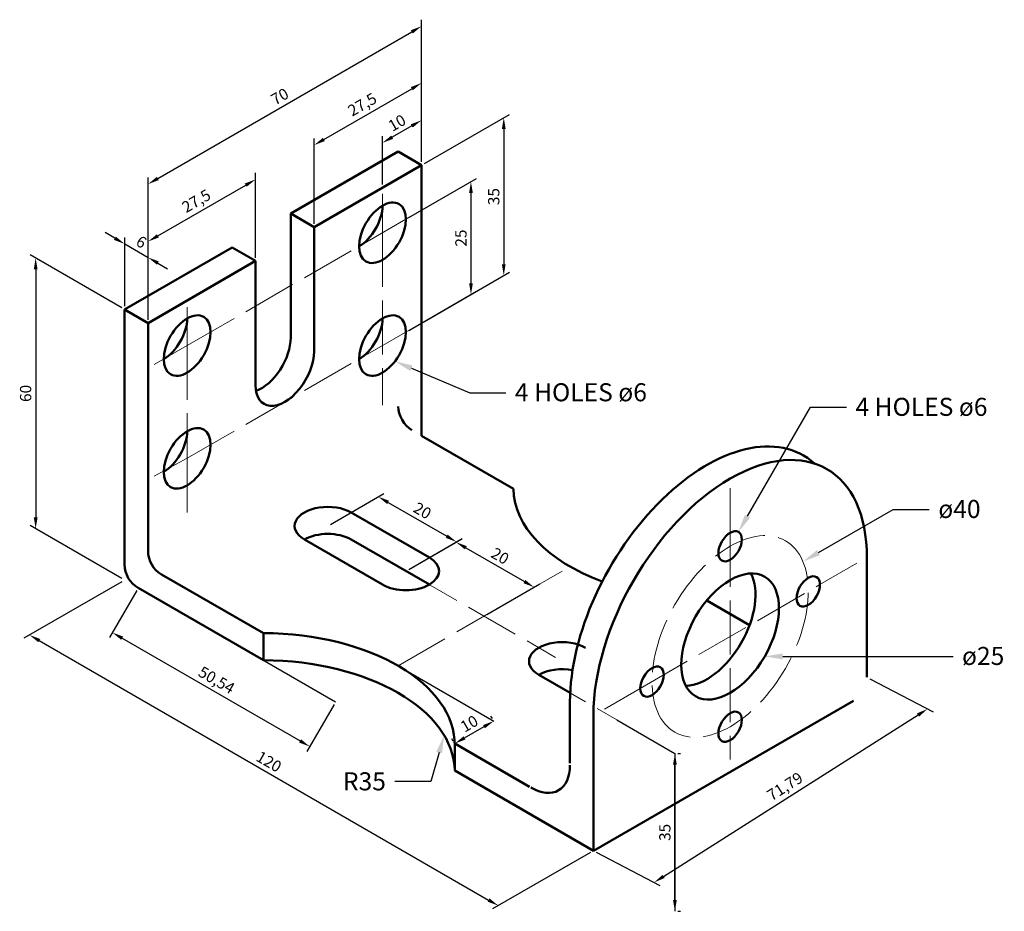
# Model space of a CAD drawing. Units: millimetres. Extents: x 1305 to 1523, y 1896 to 2094.
import ezdxf
from ezdxf import colors
from ezdxf.entities.mleader import LeaderData, LeaderLine
from ezdxf.math import Vec2, Vec3

# ---------------------------------------------------------------- set-up
doc = ezdxf.new("R2010")
doc.units = ezdxf.units.MM
doc.linetypes.add('ACAD_ISO02W100', pattern=[15, 12, -3])
for name, color, linetype, lineweight in [('M-CNTR', 1, 'ACAD_ISO02W100', 18), ('M-DIMS', 2, 'Continuous', 25), ('M-OUTL', 7, 'Continuous', 50), ('M-TEXT', 3, 'Continuous', 25)]:
    doc.layers.add(name, color=color, linetype=linetype, lineweight=lineweight)
doc.styles.get("Standard").update_dxf_attribs({"font": 'arial.ttf'})
doc.dimstyles.new('ISO-25', dxfattribs={"dimtxt": 2.5, "dimasz": 2.5, "dimexe": 1.25, "dimexo": 0.625, "dimtad": 1, "dimtxsty": 'Standard', "dimcen": 2.5, "dimadec": 0, "dimazin": 0, "dimtfac": 1, "dimtmove": 0, "dimatfit": 3, "dimfxl": 1, "dimarcsym": 0})

# ---------------------------------------------------------------- blocks, each defined once
blk = doc.blocks.new('*D1')
at = {"layer": 'Defpoints', "color": 0, "transparency": 16777216}
for p in [(1493, 1948.39), (1506.45, 1941.36), (1432.38, 1909.92)]:
    blk.add_point(p, dxfattribs=at)
at = {"layer": 'M-DIMS', "color": 0, "lineweight": -2, "transparency": 16777216}
for p, q in [((1493.64, 1948.05), (1507.73, 1940.69)), ((1447.94, 1904.23), (1504.34, 1940.02)), ((1433.02, 1909.59), (1447.11, 1902.22))]:
    blk.add_line(p, q, dxfattribs=at)
at = {"layer": 'M-DIMS', "color": 0, "transparency": 16777216}
for points in [[(1504.11, 1940.37), (1504.56, 1939.66), (1506.45, 1941.36)], [(1447.71, 1904.58), (1448.16, 1903.88), (1445.83, 1902.89)]]:
    blk.add_solid(points, dxfattribs=at)
at = {"layer": 'M-DIMS', "color": 0, "transparency": 16777216, "insert": (1475, 1923.92), "char_height": 2.5, "attachment_point": 5, "rotation": 32.3948}
blk.add_mtext('71,79', dxfattribs=at)
blk = doc.blocks.new('*D2')
at = {"layer": 'Defpoints', "color": 0, "transparency": 16777216}
for p in [(1328.46, 1969.92), (1432.38, 1909.92), (1411.29, 1897.75)]:
    blk.add_point(p, dxfattribs=at)
at = {"layer": 'M-DIMS', "color": 0, "lineweight": -2, "transparency": 16777216}
for p, q in [((1327.83, 1969.56), (1306.12, 1957.03)), ((1309.54, 1956.5), (1409.13, 1899)), ((1431.75, 1909.56), (1410.04, 1897.03))]:
    blk.add_line(p, q, dxfattribs=at)
at = {"layer": 'M-DIMS', "color": 0, "transparency": 16777216}
for points in [[(1309.75, 1956.86), (1309.33, 1956.14), (1307.37, 1957.75)], [(1409.34, 1899.36), (1408.92, 1898.64), (1411.29, 1897.75)]]:
    blk.add_solid(points, dxfattribs=at)
at = {"layer": 'M-DIMS', "color": 0, "transparency": 16777216, "insert": (1360.28, 1929.4), "char_height": 2.5, "attachment_point": 5, "rotation": 330}
blk.add_mtext('120', dxfattribs=at)
blk = doc.blocks.new('*D3')
at = {"layer": 'Defpoints', "color": 0, "transparency": 16777216}
for p in [(1328.46, 2029.92), (1308.73, 1981.31), (1328.46, 1969.92)]:
    blk.add_point(p, dxfattribs=at)
at = {"layer": 'M-DIMS', "color": 0, "lineweight": -2, "transparency": 16777216}
for p, q in [((1327.83, 2030.28), (1307.48, 2042.03)), ((1308.73, 2038.81), (1308.73, 1983.81)), ((1327.83, 1970.28), (1307.48, 1982.03))]:
    blk.add_line(p, q, dxfattribs=at)
at = {"layer": 'M-DIMS', "color": 0, "transparency": 16777216}
for points in [[(1308.31, 2038.81), (1309.15, 2038.81), (1308.73, 2041.31)], [(1308.31, 1983.81), (1309.15, 1983.81), (1308.73, 1981.31)]]:
    blk.add_solid(points, dxfattribs=at)
at = {"layer": 'M-DIMS', "color": 0, "transparency": 16777216, "insert": (1306.83, 2011.31), "char_height": 2.5, "attachment_point": 5, "rotation": 90}
blk.add_mtext('60', dxfattribs=at)
blk = doc.blocks.new('*D4')
at = {"layer": 'Defpoints', "color": 0, "transparency": 16777216}
for p in [(1333.65, 2041.46), (1328.46, 2029.92), (1333.65, 2026.92)]:
    blk.add_point(p, dxfattribs=at)
at = {"layer": 'M-DIMS', "color": 0, "lineweight": -2, "transparency": 16777216}
for p, q in [((1326.29, 2045.71), (1324.13, 2046.96)), ((1328.46, 2030.65), (1328.46, 2045.9)), ((1328.46, 2044.46), (1333.65, 2041.46)), ((1333.65, 2027.65), (1333.65, 2042.9)), ((1335.82, 2040.21), (1337.98, 2038.96))]:
    blk.add_line(p, q, dxfattribs=at)
at = {"layer": 'M-DIMS', "color": 0, "transparency": 16777216}
for points in [[(1326.5, 2046.07), (1326.08, 2045.35), (1328.46, 2044.46)], [(1336.03, 2040.57), (1335.61, 2039.85), (1333.65, 2041.46)]]:
    blk.add_solid(points, dxfattribs=at)
at = {"layer": 'M-DIMS', "color": 0, "transparency": 16777216, "insert": (1332, 2044.61), "char_height": 2.5, "attachment_point": 5, "rotation": 330}
blk.add_mtext('6', dxfattribs=at)
blk = doc.blocks.new('*D5')
at = {"layer": 'Defpoints', "color": 0, "transparency": 16777216}
for p in [(1357.47, 2058.74), (1357.47, 2040.67), (1333.65, 2026.92)]:
    blk.add_point(p, dxfattribs=at)
at = {"layer": 'M-DIMS', "color": 0, "lineweight": -2, "transparency": 16777216}
for p, q in [((1357.47, 2041.4), (1357.47, 2060.18)), ((1335.82, 2046.24), (1355.3, 2057.49)), ((1333.65, 2027.65), (1333.65, 2046.43))]:
    blk.add_line(p, q, dxfattribs=at)
at = {"layer": 'M-DIMS', "color": 0, "transparency": 16777216}
for points in [[(1355.09, 2057.85), (1355.51, 2057.13), (1357.47, 2058.74)], [(1335.61, 2046.6), (1336.03, 2045.88), (1333.65, 2044.99)]]:
    blk.add_solid(points, dxfattribs=at)
at = {"layer": 'M-DIMS', "color": 0, "transparency": 16777216, "insert": (1344.5, 2053.71), "char_height": 2.5, "attachment_point": 5, "rotation": 30}
blk.add_mtext('27,5', dxfattribs=at)
blk = doc.blocks.new('*D6')
at = {"layer": 'Defpoints', "color": 0, "transparency": 16777216}
for p in [(1394.27, 2092.72), (1394.27, 2061.92), (1333.65, 2026.92)]:
    blk.add_point(p, dxfattribs=at)
at = {"layer": 'M-DIMS', "color": 0, "lineweight": -2, "transparency": 16777216}
for p, q in [((1394.27, 2062.65), (1394.27, 2094.17)), ((1335.82, 2058.97), (1392.11, 2091.47)), ((1333.65, 2027.65), (1333.65, 2059.17))]:
    blk.add_line(p, q, dxfattribs=at)
at = {"layer": 'M-DIMS', "color": 0, "transparency": 16777216}
for points in [[(1391.9, 2091.83), (1392.32, 2091.11), (1394.27, 2092.72)], [(1335.61, 2059.33), (1336.03, 2058.61), (1333.65, 2057.72)]]:
    blk.add_solid(points, dxfattribs=at)
at = {"layer": 'M-DIMS', "color": 0, "transparency": 16777216, "insert": (1363.01, 2076.87), "char_height": 2.5, "attachment_point": 5, "rotation": 30}
blk.add_mtext('70', dxfattribs=at)
blk = doc.blocks.new('*D7')
at = {"layer": 'Defpoints', "color": 0, "transparency": 16777216}
for p in [(1385.61, 2066.87), (1394.27, 2061.92), (1385.61, 2056.92)]:
    blk.add_point(p, dxfattribs=at)
at = {"layer": 'M-DIMS', "color": 0, "lineweight": -2, "transparency": 16777216}
for p, q in [((1394.27, 2062.65), (1394.27, 2073.31)), ((1392.11, 2070.62), (1387.78, 2068.12)), ((1385.61, 2057.65), (1385.61, 2068.31))]:
    blk.add_line(p, q, dxfattribs=at)
at = {"layer": 'M-DIMS', "color": 0, "transparency": 16777216}
for points in [[(1391.9, 2070.98), (1392.32, 2070.26), (1394.27, 2071.87)], [(1387.57, 2068.48), (1387.99, 2067.76), (1385.61, 2066.87)]]:
    blk.add_solid(points, dxfattribs=at)
at = {"layer": 'M-DIMS', "color": 0, "transparency": 16777216, "insert": (1388.99, 2071.02), "char_height": 2.5, "attachment_point": 5, "rotation": 30}
blk.add_mtext('10', dxfattribs=at)
blk = doc.blocks.new('*D8')
at = {"layer": 'Defpoints', "color": 0, "transparency": 16777216}
for p in [(1394.27, 2080.12), (1394.27, 2061.92), (1370.46, 2048.17)]:
    blk.add_point(p, dxfattribs=at)
at = {"layer": 'M-DIMS', "color": 0, "lineweight": -2, "transparency": 16777216}
for p, q in [((1394.27, 2062.65), (1394.27, 2081.57)), ((1372.62, 2067.62), (1392.11, 2078.87)), ((1370.46, 2048.9), (1370.46, 2067.82))]:
    blk.add_line(p, q, dxfattribs=at)
at = {"layer": 'M-DIMS', "color": 0, "transparency": 16777216}
for points in [[(1391.9, 2079.23), (1392.32, 2078.51), (1394.27, 2080.12)], [(1372.42, 2067.98), (1372.83, 2067.26), (1370.46, 2066.37)]]:
    blk.add_solid(points, dxfattribs=at)
at = {"layer": 'M-DIMS', "color": 0, "transparency": 16777216, "insert": (1381.3, 2075.09), "char_height": 2.5, "attachment_point": 5, "rotation": 30}
blk.add_mtext('27,5', dxfattribs=at)
blk = doc.blocks.new('*D9')
at = {"layer": 'Defpoints', "color": 0, "transparency": 16777216}
for p in [(1390.81, 2049.92), (1405.23, 2033.25), (1390.81, 2024.92)]:
    blk.add_point(p, dxfattribs=at)
at = {"layer": 'M-DIMS', "color": 0, "lineweight": -2, "transparency": 16777216}
for p, q in [((1391.43, 2050.28), (1406.48, 2058.97)), ((1405.23, 2055.75), (1405.23, 2035.75)), ((1391.43, 2025.28), (1406.48, 2033.97))]:
    blk.add_line(p, q, dxfattribs=at)
at = {"layer": 'M-DIMS', "color": 0, "transparency": 16777216}
for points in [[(1404.81, 2055.75), (1405.65, 2055.75), (1405.23, 2058.25)], [(1404.81, 2035.75), (1405.65, 2035.75), (1405.23, 2033.25)]]:
    blk.add_solid(points, dxfattribs=at)
at = {"layer": 'M-DIMS', "color": 0, "transparency": 16777216, "insert": (1403.33, 2045.75), "char_height": 2.5, "attachment_point": 5, "rotation": 90}
blk.add_mtext('25', dxfattribs=at)
blk = doc.blocks.new('*D10')
at = {"layer": 'Defpoints', "color": 0, "transparency": 16777216}
for p in [(1394.27, 2061.92), (1412.5, 2037.45), (1394.27, 2026.92)]:
    blk.add_point(p, dxfattribs=at)
at = {"layer": 'M-DIMS', "color": 0, "lineweight": -2, "transparency": 16777216}
for p, q in [((1394.9, 2062.28), (1413.75, 2073.17)), ((1412.5, 2069.95), (1412.5, 2039.95)), ((1394.9, 2027.28), (1413.75, 2038.17))]:
    blk.add_line(p, q, dxfattribs=at)
at = {"layer": 'M-DIMS', "color": 0, "transparency": 16777216}
for points in [[(1412.09, 2069.95), (1412.92, 2069.95), (1412.5, 2072.45)], [(1412.09, 2039.95), (1412.92, 2039.95), (1412.5, 2037.45)]]:
    blk.add_solid(points, dxfattribs=at)
at = {"layer": 'M-DIMS', "color": 0, "transparency": 16777216, "insert": (1410.6, 2054.95), "char_height": 2.5, "attachment_point": 5, "rotation": 90}
blk.add_mtext('35', dxfattribs=at)
blk = doc.blocks.new('*D11')
at = {"layer": 'Defpoints', "color": 0, "transparency": 16777216}
for p in [(1373.49, 1981.92), (1402.02, 1978.4), (1390.81, 1971.92)]:
    blk.add_point(p, dxfattribs=at)
at = {"layer": 'M-DIMS', "color": 0, "lineweight": -2, "transparency": 16777216}
for p, q in [((1374.11, 1982.28), (1385.95, 1989.12)), ((1386.86, 1987.15), (1399.85, 1979.65)), ((1391.43, 1972.28), (1403.27, 1979.12))]:
    blk.add_line(p, q, dxfattribs=at)
at = {"layer": 'M-DIMS', "color": 0, "transparency": 16777216}
for points in [[(1387.07, 1987.51), (1386.66, 1986.78), (1384.7, 1988.4)], [(1400.06, 1980.01), (1399.65, 1979.28), (1402.02, 1978.4)]]:
    blk.add_solid(points, dxfattribs=at)
at = {"layer": 'M-DIMS', "color": 0, "transparency": 16777216, "insert": (1394.31, 1985.04), "char_height": 2.5, "attachment_point": 5, "rotation": 330}
blk.add_mtext('20', dxfattribs=at)
blk = doc.blocks.new('*D12')
at = {"layer": 'Defpoints', "color": 0, "transparency": 16777216}
for p in [(1390.81, 1971.92), (1419.24, 1968.34), (1408.13, 1961.92)]:
    blk.add_point(p, dxfattribs=at)
at = {"layer": 'M-DIMS', "color": 0, "lineweight": -2, "transparency": 16777216}
for p, q in [((1391.43, 1972.28), (1403.17, 1979.06)), ((1404.09, 1977.09), (1417.08, 1969.59)), ((1408.76, 1962.28), (1420.49, 1969.06))]:
    blk.add_line(p, q, dxfattribs=at)
at = {"layer": 'M-DIMS', "color": 0, "transparency": 16777216}
for points in [[(1404.3, 1977.45), (1403.88, 1976.73), (1401.92, 1978.34)], [(1417.29, 1969.95), (1416.87, 1969.23), (1419.24, 1968.34)]]:
    blk.add_solid(points, dxfattribs=at)
at = {"layer": 'M-DIMS', "color": 0, "transparency": 16777216, "insert": (1411.53, 1974.99), "char_height": 2.5, "attachment_point": 5, "rotation": 330}
blk.add_mtext('20', dxfattribs=at)
blk = doc.blocks.new('*D13')
at = {"layer": 'Defpoints', "color": 0, "transparency": 16777216}
for p in [(1410.29, 1938.68), (1410.29, 1938.68), (1401.63, 1933.68)]:
    blk.add_point(p, dxfattribs=at)
at = {"layer": 'M-DIMS', "color": 0, "lineweight": -2, "transparency": 16777216}
for p, q in [((1409.98, 1939.22), (1409.67, 1939.76)), ((1403.8, 1934.93), (1408.13, 1937.43)), ((1401.32, 1934.22), (1401.01, 1934.76))]:
    blk.add_line(p, q, dxfattribs=at)
at = {"layer": 'M-DIMS', "color": 0, "transparency": 16777216}
for points in [[(1407.92, 1937.79), (1408.33, 1937.07), (1410.29, 1938.68)], [(1403.59, 1935.29), (1404, 1934.57), (1401.63, 1933.68)]]:
    blk.add_solid(points, dxfattribs=at)
at = {"layer": 'M-DIMS', "color": 0, "transparency": 16777216, "insert": (1405.01, 1937.82), "char_height": 2.5, "attachment_point": 5, "rotation": 30}
blk.add_mtext('10', dxfattribs=at)
blk = doc.blocks.new('*D14')
at = {"layer": 'Defpoints', "color": 0, "transparency": 16777216}
for p in [(1331.46, 1968.19), (1375.22, 1942.92), (1369.5, 1933.02)]:
    blk.add_point(p, dxfattribs=at)
at = {"layer": 'M-DIMS', "color": 0, "lineweight": -2, "transparency": 16777216}
for p, q in [((1331.14, 1967.65), (1325.11, 1957.2)), ((1327.9, 1957.04), (1367.34, 1934.27)), ((1374.91, 1942.38), (1368.88, 1931.94))]:
    blk.add_line(p, q, dxfattribs=at)
at = {"layer": 'M-DIMS', "color": 0, "transparency": 16777216}
for points in [[(1328.11, 1957.4), (1327.69, 1956.68), (1325.74, 1958.29)], [(1367.55, 1934.63), (1367.13, 1933.91), (1369.5, 1933.02)]]:
    blk.add_solid(points, dxfattribs=at)
at = {"layer": 'M-DIMS', "color": 0, "transparency": 16777216, "insert": (1348.68, 1947.49), "char_height": 2.5, "attachment_point": 5, "rotation": 330}
blk.add_mtext('50,54', dxfattribs=at)
blk = doc.blocks.new('*D15')
at = {"layer": 'Defpoints', "color": 0, "transparency": 16777216}
for p in [(1450.44, 1931.49), (1450.44, 1931.49), (1450.44, 1896.49)]:
    blk.add_point(p, dxfattribs=at)
at = {"layer": 'M-DIMS', "color": 0, "lineweight": -2, "transparency": 16777216}
for p, q in [((1451.07, 1931.49), (1451.69, 1931.49)), ((1450.44, 1898.99), (1450.44, 1928.99)), ((1451.07, 1896.49), (1451.69, 1896.49))]:
    blk.add_line(p, q, dxfattribs=at)
at = {"layer": 'M-DIMS', "color": 0, "transparency": 16777216}
for points in [[(1450.03, 1928.99), (1450.86, 1928.99), (1450.44, 1931.49)], [(1450.03, 1898.99), (1450.86, 1898.99), (1450.44, 1896.49)]]:
    blk.add_solid(points, dxfattribs=at)
at = {"layer": 'M-DIMS', "color": 0, "transparency": 16777216, "insert": (1448.54, 1913.99), "char_height": 2.5, "attachment_point": 5, "rotation": 90}
blk.add_mtext('35', dxfattribs=at)

msp = doc.modelspace()

# ---------------------------------------------------------------- linework, layer by layer
at = {"layer": 'M-CNTR'}
for p, q in [((1385.614, 2046.923), (1385.614, 2055.554)), ((1342.313, 2021.923), (1392.613, 2050.965)), ((1385.614, 2046.923), (1385.614, 2008.718)), ((1342.313, 2021.923), (1342.313, 2030.459)), ((1342.313, 1996.923), (1392.933, 2026.149)), ((1342.313, 2021.923), (1334.982, 2017.691)), ((1342.313, 2021.923), (1342.313, 1996.923)), ((1342.313, 1996.923), (1334.974, 1992.94)), ((1342.313, 1996.923), (1342.313, 1983.994)), ((1462.69, 1980.423), (1462.69, 1990.296)), ((1462.69, 1980.423), (1462.69, 1934.423)), ((1378.686, 1978.923), (1423.979, 1952.773)), ((1482.609, 1968.923), (1490.784, 1973.644)), ((1389.078, 1950.923), (1427.183, 1972.923)), ((1442.771, 1945.923), (1482.609, 1968.923)), ((1420.255, 1948.923), (1437.575, 1938.923)), ((1442.771, 1945.923), (1434.84, 1941.344)), ((1462.69, 1934.423), (1462.69, 1930.187))]:
    msp.add_line(p, q, dxfattribs=at)
msp.add_ellipse((1462.69, 1957.423), major_axis=(-12.247, -21.213), ratio=0.5773503, dxfattribs=at)
at = {"layer": 'M-DIMS'}
for p, q in [((1331.456, 1968.191), (1375.221, 1942.923)), ((1389.078, 1950.923), (1410.291, 1938.676)), ((1437.575, 1938.923), (1450.442, 1931.495)), ((1450.442, 1931.495), (1450.442, 1896.495))]:
    msp.add_line(p, q, dxfattribs=at)
at = {"layer": 'M-OUTL'}
for p, q in [((1389.078, 2064.923), (1365.262, 2051.173)), ((1365.262, 2051.173), (1389.078, 2064.923)), ((1389.078, 2064.923), (1394.274, 2061.923)), ((1370.458, 2048.173), (1394.274, 2061.923)), ((1394.274, 2061.923), (1394.274, 2001.923)), ((1394.274, 2061.923), (1394.274, 2026.923)), ((1365.262, 2051.173), (1370.458, 2048.173)), ((1365.262, 2051.173), (1365.262, 2023.673)), ((1370.458, 2048.173), (1370.458, 2020.673)), ((1328.456, 2029.923), (1352.272, 2043.673)), ((1328.456, 2029.923), (1352.272, 2043.673)), ((1328.456, 2029.923), (1352.272, 2043.673)), ((1352.272, 2043.673), (1357.468, 2040.673)), ((1333.652, 2026.923), (1357.468, 2040.673)), ((1357.468, 2040.673), (1357.468, 2013.173)), ((1328.456, 1973.388), (1328.456, 2029.923)), ((1328.456, 2029.923), (1333.652, 2026.923)), ((1333.652, 2026.923), (1333.652, 1976.388)), ((1333.652, 2026.923), (1333.652, 1991.923)), ((1394.274, 2001.923), (1414.63, 1990.171)), ((1328.456, 1973.388), (1328.456, 1985.923)), ((1378.686, 1984.923), (1396.006, 1974.923)), ((1368.293, 1978.923), (1385.614, 1968.923)), ((1378.686, 1978.923), (1396.006, 1968.923)), ((1328.456, 1973.388), (1328.456, 1975.923)), ((1493.001, 1948.388), (1493.001, 1974.923)), ((1336.652, 1971.191), (1359.204, 1958.171)), ((1331.456, 1968.191), (1359.204, 1952.171)), ((1331.456, 1968.191), (1359.204, 1952.171)), ((1457.513, 1965.412), (1467.001, 1959.935)), ((1359.204, 1958.171), (1359.204, 1952.171)), ((1420.255, 1948.923), (1427.23, 1944.896)), ((1427.183, 1929.316), (1427.183, 1942.923)), ((1432.379, 1909.923), (1490.001, 1943.191)), ((1432.379, 1939.923), (1432.379, 1909.923)), ((1401.631, 1933.676), (1401.631, 1927.676)), ((1401.631, 1933.676), (1418.183, 1924.12)), ((1432.379, 1909.923), (1401.631, 1927.676))]:
    msp.add_line(p, q, dxfattribs=at)
for centre in [(1339.652, 1976.388), (1334.456, 1973.388)]:
    msp.add_arc(centre, 6, 180, 240, dxfattribs=at)
for centre, major_axis in [((1385.614, 2046.923), (-3.674, -6.364)), ((1385.614, 2046.923), (-3.674, -6.364)), ((1342.313, 2021.923), (-3.674, -6.364)), ((1385.614, 2021.923), (-3.674, -6.364)), ((1342.313, 1996.923), (-3.674, -6.364)), ((1462.69, 1977.423), (-1.837, -3.182)), ((1462.69, 1957.423), (-7.655, -13.258)), ((1480.011, 1967.423), (-1.837, -3.182)), ((1445.37, 1947.423), (-1.837, -3.182)), ((1462.69, 1937.423), (-1.837, -3.182))]:
    msp.add_ellipse(centre, major_axis=major_axis, ratio=0.5773503, dxfattribs=at)
for centre, major_axis, start_param, end_param in [((1380.418, 2049.923), (3.674, 6.364), 3.9269908, 5.4977871), ((1337.116, 2024.923), (3.674, 6.364), 3.9269908, 5.4977871), ((1380.418, 2024.923), (3.674, 6.364), 3.9269908, 5.4977871), ((1358.767, 2019.923), (-4.593, -7.955), 6.8844495, 8.6393798), ((1363.963, 2016.923), (-4.593, -7.955), 5.4977871, 8.6393798), ((1392.109, 2006.673), (-2.143, 3.712), 0.7853982, 2.3561945), ((1337.116, 1999.923), (3.674, 6.364), 3.9269908, 5.4977871), ((1457.494, 1960.423), (-21.433, -37.123), 3.0200755, 5.4977871), ((1462.69, 1957.423), (-21.433, -37.123), 2.3561945, 5.4977871), ((1457.494, 1990.423), (-42.866, 0), 6.2933901, 7.2828042), ((1373.489, 1981.923), (-7.348, 0), 3.9269908, 7.0685835), ((1373.489, 1975.923), (-7.348, 0), 3.9269908, 5.4977871), ((1390.81, 1971.923), (-7.348, 0), 0.7853982, 3.9269908), ((1457.494, 1960.423), (-7.655, -13.258), 6.6294762, 9.078487), ((1358.767, 1933.423), (-42.866, 0), 3.1313879, 4.7021842), ((1425.451, 1951.923), (-7.348, 0), 3.9269908, 7.0685835), ((1358.767, 1927.423), (-42.866, 0), 9.4349828, 10.9853695), ((1425.451, 1945.923), (-7.348, 0), 4.3949534, 5.4977871), ((1457.494, 1960.423), (-7.655, -13.258), 5.9926059, 5.9984419), ((1418.523, 1933.923), (-6.124, 10.607), 3.1415927, 3.9269908), ((1418.523, 1933.923), (-6.124, 10.607), 2.3561945, 3.1415927)]:
    msp.add_ellipse(centre, major_axis=major_axis, ratio=0.5773503, start_param=start_param, end_param=end_param, dxfattribs=at)

# ---------------------------------------------------------------- dimensions: what is measured, and where the dimension line sits
at = {"layer": 'M-DIMS'}
for p1, p2, distance, picture, middle in [((1333.652, 2026.923), (1394.274, 2061.923), 26.674, '*D6', (1363.012, 2076.87)), ((1370.458, 2048.173), (1394.274, 2061.923), 15.76, '*D8', (1381.303, 2075.089)), ((1394.274, 2061.923), (1385.614, 2056.923), -8.615, '*D7', (1388.993, 2071.017)), ((1394.274, 2061.923), (1394.274, 2026.923), 18.23, '*D10', (1410.602, 2054.949)), ((1333.652, 2026.923), (1357.468, 2040.673), 15.645, '*D5', (1344.496, 2053.706)), ((1390.81, 2049.923), (1390.81, 2024.923), 14.421, '*D9', (1403.33, 2045.75)), ((1328.456, 2029.923), (1333.652, 2026.923), 12.589, '*D4', (1332.005, 2044.607)), ((1328.456, 2029.923), (1328.456, 1969.923), -19.727, '*D3', (1306.828, 2011.313)), ((1373.489, 1981.923), (1390.81, 1971.923), 11.21, '*D11', (1394.31, 1985.042)), ((1390.81, 1971.923), (1408.13, 1961.923), 11.112, '*D12', (1411.533, 1974.986)), ((1328.456, 1969.923), (1432.379, 1909.923), -21.084, '*D2', (1360.284, 1929.397)), ((1432.3792, 1909.9235), (1493.001, 1948.3876), -13.1419, '*D1', (1474.9977, 1923.9201)), ((1401.631, 1933.676), (1410.291, 1938.676), 0, '*D13', (1405.01, 1937.823))]:
    dim = msp.add_aligned_dim(p1=p1, p2=p2, distance=distance, dimstyle='ISO-25', override={"dimclrd": 0, "dimclre": 0, "dimclrt": 0}, dxfattribs=at)
    dim.commit()
    dim.dimension.update_dxf_attribs({"geometry": picture, "text_midpoint": middle})
for base, p1, p2, angle, picture, middle in [((1369.503, 1933.018), (1331.456, 1968.191), (1375.221, 1942.923), 330, '*D14', (1348.684, 1947.495)), ((1450.442, 1931.495), (1450.442, 1896.495), (1450.442, 1931.495), 90, '*D15', (1448.54, 1913.995))]:
    dim = msp.add_linear_dim(base=base, p1=p1, p2=p2, angle=angle, dimstyle='ISO-25', override={"dimrnd": 0}, dxfattribs=at)
    dim.commit()
    dim.dimension.update_dxf_attribs({"geometry": picture, "text_midpoint": middle})

# ---------------------------------------------------------------- leaders
at = {"layer": 'M-TEXT'}
ml = msp.add_multileader_mtext('Standard', dxfattribs=at)
ml.set_content('4 HOLES ø6', color=256)
ml.set_leader_properties()
ml.build(insert=Vec2(0, 0))
ctx = ml.context
ctx.base_point, ctx.plane_origin = Vec3(1412.973, 2011.46), Vec3(1388.372, 2018.431)
notes = []
notes.append((ctx, [(0, (1, 1, 0), (1404.973, 2011.46), (1, 0), 8, [(0, [(1388.372, 2018.431)], 0, [])])]))
ctx.mtext.insert, ctx.mtext.flow_direction = Vec3(1414.973, 2013.568), 5
ml = msp.add_multileader_mtext('Standard', dxfattribs=at)
ml.set_content('4 HOLES ø6', color=256)
ml.set_leader_properties()
ml.build(insert=Vec2(0, 0))
ctx = ml.context
ctx.base_point, ctx.plane_origin = Vec3(1488.475, 2008.229), Vec3(1464.527, 1980.605)
notes.append((ctx, [(0, (1, 1, 0), (1480.475, 2008.229), (1, 0), 8, [(0, [(1464.527, 1980.605)], 0, [])])]))
ctx.mtext.insert, ctx.mtext.flow_direction = Vec3(1490.475, 2010.336), 5
ml = msp.add_multileader_mtext('Standard', dxfattribs=at)
ml.set_content('ø40', color=256)
ml.set_leader_properties()
ml.build(insert=Vec2(0, 0))
ctx = ml.context
ctx.base_point, ctx.plane_origin = Vec3(1506.843, 1985.587), Vec3(1478.819, 1974.026)
notes.append((ctx, [(0, (1, 1, 0), (1498.843, 1985.587), (1, 0), 8, [(0, [(1478.819, 1974.026)], 0, [])])]))
ctx.mtext.insert, ctx.mtext.flow_direction = Vec3(1508.843, 1987.694), 5
ml = msp.add_multileader_mtext('Standard', dxfattribs=at)
ml.set_content('ø25', color=256)
ml.set_leader_properties()
ml.build(insert=Vec2(0, 0))
ctx = ml.context
ctx.base_point, ctx.plane_origin = Vec3(1512.105, 1953.004), Vec3(1470.345, 1953.004)
notes.append((ctx, [(0, (1, 1, 0), (1504.105, 1953.004), (1, 0), 8, [(0, [(1470.345, 1953.004)], 0, [])])]))
ctx.mtext.insert, ctx.mtext.flow_direction = Vec3(1514.105, 1955.112), 5
ml = msp.add_multileader_mtext('Standard', dxfattribs=at)
ml.set_content('R35', color=256)
ml.set_leader_properties()
ml.build(insert=Vec2(0, 0))
ctx = ml.context
ctx.base_point, ctx.plane_origin = Vec3(1374.783, 1925.275), Vec3(1399.273, 1935.522)
ctx.text_align_type = 2
notes.append((ctx, [(0, (1, 1, 0), (1396.371, 1925.275), (-1, 0), 8, [(0, [(1399.273, 1935.522)], 0, [])])]))
ctx.mtext.insert, ctx.mtext.alignment, ctx.mtext.flow_direction = Vec3(1386.371, 1927.31), 3, 5
for ctx, leaders in notes:
    for number, flags, end, landing, length, lines in leaders:
        leader = LeaderData()
        leader.index, (leader.has_last_leader_line, leader.has_dogleg_vector, leader.attachment_direction) = number, flags
        leader.last_leader_point, leader.dogleg_vector, leader.dogleg_length = Vec3(end), Vec3(landing), length
        for number, points, colour, breaks in lines:
            line = LeaderLine()
            line.index, line.vertices, line.color, line.breaks = number, Vec3.list(points), colors.encode_raw_color(colour), breaks
            leader.lines.append(line)
        ctx.leaders.append(leader)

doc.saveas('drawing.dxf')
